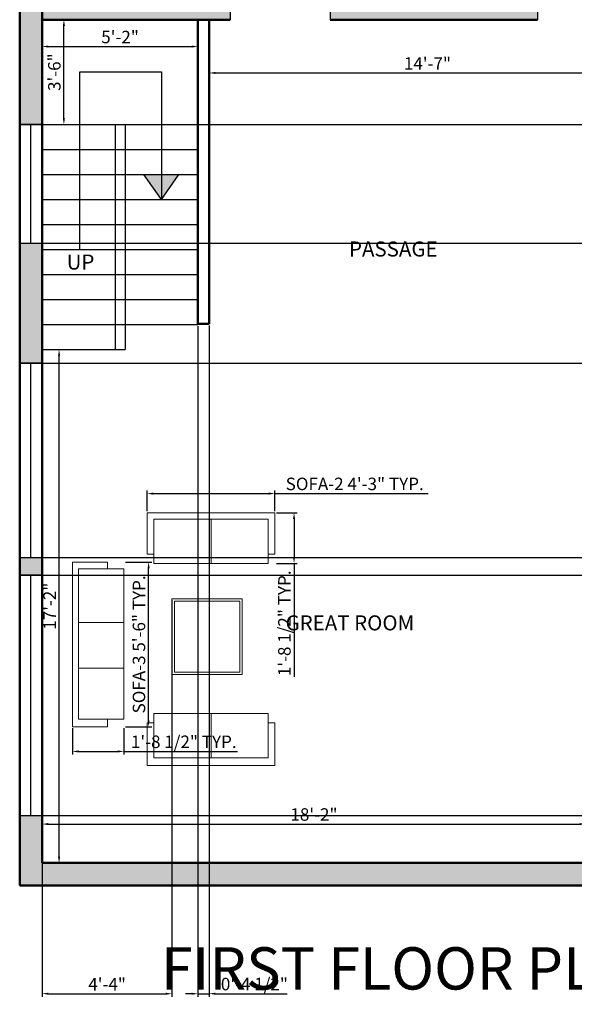
# Model space of a CAD drawing. Units: inches. Extents: x 2064 to 2999, y 1440 to 2089.
# Tile 5 of 7: x 2541 to 2763, y 1440 to 1835. Entities that reach past the tile are written whole.
import ezdxf

# ---------------------------------------------------------------- set-up
doc = ezdxf.new("R2010")
doc.units = ezdxf.units.IN
for name, color, linetype, lineweight in [('A-ANNO-DIMS', 2, 'Continuous', 18), ('A-ANNO-TEXT', 3, 'Continuous', 18), ('A-AREA-IDEN', 7, 'Continuous', 18), ('A-DOOR', 4, 'Continuous', 25), ('A-FLOR-STRS', 2, 'Continuous', 25), ('A-FURN', 8, 'Continuous', 18), ('A-GLAZ', 3, 'Continuous', 25), ('A-WALL', 7, 'Continuous', 50), ('A-WALL-PATT', 8, 'Continuous', 13)]:
    doc.layers.add(name, color=color, linetype=linetype, lineweight=lineweight)
doc.styles.get("Standard").update_dxf_attribs({"font": 'arial.ttf'})
doc.dimstyles.new('ISO-25', dxfattribs={"dimtxt": 5, "dimasz": 2.5, "dimexe": 1.25, "dimexo": 0.625, "dimtad": 1, "dimdec": 0, "dimlunit": 4, "dimtxsty": 'Standard', "dimcen": 2.5, "dimadec": 0, "dimazin": 0, "dimtfac": 1, "dimtdec": 0, "dimtmove": 0, "dimatfit": 3, "dimfxl": 1, "dimarcsym": 0})

# ---------------------------------------------------------------- blocks, each defined once
blk = doc.blocks.new('*U2')
for p, q in [((0, 0), (0, -6)), ((40, 0), (40, -6))]:
    blk.add_line(p, q)
blk.add_lwpolyline([(0, 0), (0, 40), (1.75, 40), (1.75, 0)], close=True)
blk.add_arc((0, 0), 40, 0, 90)
blk = doc.blocks.new('*D31')
at = {"layer": 'A-ANNO-DIMS', "color": 0, "lineweight": -2, "transparency": 16777216}
for p, q in [((2549.87, 1497.7), (2549.87, 1513.87)), ((2767.37, 1497.7), (2767.37, 1513.87)), ((2552.37, 1512.62), (2764.87, 1512.62))]:
    blk.add_line(p, q, dxfattribs=at)
at = {"layer": 'A-ANNO-DIMS', "color": 0, "transparency": 16777216}
for points in [[(2552.37, 1513.04), (2552.37, 1512.2), (2549.87, 1512.62)], [(2764.87, 1513.04), (2764.87, 1512.2), (2767.37, 1512.62)]]:
    blk.add_solid(points, dxfattribs=at)
at = {"layer": 'Defpoints', "color": 0, "transparency": 16777216}
for p in [(2767.37, 1512.62), (2549.87, 1497.07), (2767.37, 1497.07)]:
    blk.add_point(p, dxfattribs=at)
at = {"layer": 'A-ANNO-DIMS', "color": 0, "transparency": 16777216, "insert": (2658.62, 1515.8), "char_height": 5, "attachment_point": 5}
blk.add_mtext('18\'-2"', dxfattribs=at)
blk = doc.blocks.new('*D32')
at = {"layer": 'A-ANNO-DIMS', "color": 0, "lineweight": -2, "transparency": 16777216}
for p, q in [((2550.5, 1702.57), (2557.87, 1702.57)), ((2556.62, 1499.57), (2556.62, 1700.07)), ((2550.5, 1497.07), (2557.87, 1497.07))]:
    blk.add_line(p, q, dxfattribs=at)
at = {"layer": 'A-ANNO-DIMS', "color": 0, "transparency": 16777216}
for points in [[(2556.21, 1700.07), (2557.04, 1700.07), (2556.62, 1702.57)], [(2556.21, 1499.57), (2557.04, 1499.57), (2556.62, 1497.07)]]:
    blk.add_solid(points, dxfattribs=at)
at = {"layer": 'Defpoints', "color": 0, "transparency": 16777216}
for p in [(2549.87, 1702.57), (2556.62, 1702.57), (2549.87, 1497.07)]:
    blk.add_point(p, dxfattribs=at)
at = {"layer": 'A-ANNO-DIMS', "color": 0, "transparency": 16777216, "insert": (2553.49, 1599.82), "char_height": 5, "attachment_point": 5, "rotation": 90}
blk.add_mtext('17\'-2"', dxfattribs=at)
blk = doc.blocks.new('*D33')
at = {"layer": 'A-ANNO-DIMS', "color": 0, "lineweight": -2, "transparency": 16777216}
for p, q in [((2616.69, 1833.95), (2616.69, 1812)), ((2791.37, 1833.95), (2791.37, 1812)), ((2619.19, 1813.25), (2788.87, 1813.25))]:
    blk.add_line(p, q, dxfattribs=at)
at = {"layer": 'A-ANNO-DIMS', "color": 0, "transparency": 16777216}
for points in [[(2619.19, 1813.67), (2619.19, 1812.84), (2616.69, 1813.25)], [(2788.87, 1813.67), (2788.87, 1812.84), (2791.37, 1813.25)]]:
    blk.add_solid(points, dxfattribs=at)
at = {"layer": 'Defpoints', "color": 0, "transparency": 16777216}
for p in [(2616.69, 1834.57), (2791.37, 1834.57), (2791.37, 1813.25)]:
    blk.add_point(p, dxfattribs=at)
at = {"layer": 'A-ANNO-DIMS', "color": 0, "transparency": 16777216, "insert": (2704.03, 1816.39), "char_height": 5, "attachment_point": 5}
blk.add_mtext('14\'-7"', dxfattribs=at)
blk = doc.blocks.new('*D34')
at = {"layer": 'A-ANNO-DIMS', "color": 0, "lineweight": -2, "transparency": 16777216}
for p, q in [((2549.87, 1833.95), (2549.87, 1822.57)), ((2612.19, 1833.95), (2612.19, 1822.57)), ((2552.37, 1823.82), (2609.69, 1823.82))]:
    blk.add_line(p, q, dxfattribs=at)
at = {"layer": 'A-ANNO-DIMS', "color": 0, "transparency": 16777216}
for points in [[(2552.37, 1824.24), (2552.37, 1823.4), (2549.87, 1823.82)], [(2609.69, 1824.24), (2609.69, 1823.4), (2612.19, 1823.82)]]:
    blk.add_solid(points, dxfattribs=at)
at = {"layer": 'Defpoints', "color": 0, "transparency": 16777216}
for p in [(2549.87, 1834.57), (2612.19, 1834.57), (2612.19, 1823.82)]:
    blk.add_point(p, dxfattribs=at)
at = {"layer": 'A-ANNO-DIMS', "color": 0, "transparency": 16777216, "insert": (2581.03, 1827), "char_height": 5, "attachment_point": 5}
blk.add_mtext('5\'-2"', dxfattribs=at)
blk = doc.blocks.new('*D35')
at = {"layer": 'A-ANNO-DIMS', "color": 0, "lineweight": -2, "transparency": 16777216}
for p, q in [((2550.5, 1834.57), (2559.81, 1834.57)), ((2558.56, 1795.07), (2558.56, 1832.07)), ((2550.5, 1792.57), (2559.81, 1792.57))]:
    blk.add_line(p, q, dxfattribs=at)
at = {"layer": 'A-ANNO-DIMS', "color": 0, "transparency": 16777216}
for points in [[(2558.15, 1832.07), (2558.98, 1832.07), (2558.56, 1834.57)], [(2558.15, 1795.07), (2558.98, 1795.07), (2558.56, 1792.57)]]:
    blk.add_solid(points, dxfattribs=at)
at = {"layer": 'Defpoints', "color": 0, "transparency": 16777216}
for p in [(2549.87, 1834.57), (2558.56, 1834.57), (2549.87, 1792.57)]:
    blk.add_point(p, dxfattribs=at)
at = {"layer": 'A-ANNO-DIMS', "color": 0, "transparency": 16777216, "insert": (2555.38, 1813.57), "char_height": 5, "attachment_point": 5, "rotation": 90}
blk.add_mtext('3\'-6"', dxfattribs=at)
blk = doc.blocks.new('SOFA-2')
for p, q in [((25.58, 20.31), (25.58, 2.6)), ((2.71, 16.54), (0, 16.54)), ((0, 16.54), (0, 0)), ((51.13, 16.54), (48.46, 16.54)), ((51.13, 0), (51.13, 16.54)), ((0, 0), (51.13, 0))]:
    blk.add_line(p, q)
blk.add_lwpolyline([(2.71, 2.6), (48.46, 2.6), (48.46, 20.31), (2.71, 20.31)], close=True)
blk = doc.blocks.new('SOFA-3')
for p, q in [((0, 0), (0, 65.92)), ((0, 65.92), (14.01, 65.92)), ((14.01, 65.92), (14.01, 63.25)), ((20.61, 41.74), (2.39, 41.74)), ((20.61, 23.49), (2.39, 23.49)), ((14.01, 3.1), (14.01, 0)), ((14.01, 0), (0, 0))]:
    blk.add_line(p, q)
blk.add_lwpolyline([(2.39, 3.1), (20.61, 3.1), (20.61, 63.25), (2.39, 63.25)], close=True)
blk = doc.blocks.new('COFFEE-TABLE')
for points in [[(0, 0), (28.15, 0), (28.15, 30.4), (0, 30.4)], [(1, 1), (27.15, 1), (27.15, 29.4), (1, 29.4)]]:
    blk.add_lwpolyline(points, close=True)
blk = doc.blocks.new('*D51')
at = {"layer": 'A-ANNO-DIMS', "color": 0, "lineweight": -2, "transparency": 16777216}
for p, q in [((2591.86, 1637.86), (2591.86, 1646.15)), ((2594.36, 1644.9), (2640.49, 1644.9)), ((2642.99, 1637.86), (2642.99, 1646.15)), ((2642.99, 1644.9), (2704.36, 1644.9))]:
    blk.add_line(p, q, dxfattribs=at)
at = {"layer": 'A-ANNO-DIMS', "color": 0, "transparency": 16777216}
for points in [[(2594.36, 1645.32), (2594.36, 1644.49), (2591.86, 1644.9)], [(2640.49, 1645.32), (2640.49, 1644.49), (2642.99, 1644.9)]]:
    blk.add_solid(points, dxfattribs=at)
at = {"layer": 'Defpoints', "color": 0, "transparency": 16777216}
for p in [(2642.99, 1644.9), (2591.86, 1637.24), (2642.99, 1637.24)]:
    blk.add_point(p, dxfattribs=at)
at = {"layer": 'A-ANNO-DIMS', "color": 0, "transparency": 16777216, "insert": (2674.92, 1648.12), "char_height": 5, "attachment_point": 5}
blk.add_mtext('SOFA-2 4\'-3" TYP.', dxfattribs=at)
blk = doc.blocks.new('*D52')
at = {"layer": 'A-ANNO-DIMS', "color": 0, "lineweight": -2, "transparency": 16777216}
for p, q in [((2643.61, 1637.24), (2651.9, 1637.24)), ((2650.65, 1634.74), (2650.65, 1619.43)), ((2643.61, 1616.93), (2651.9, 1616.93)), ((2650.65, 1616.93), (2650.65, 1571.52))]:
    blk.add_line(p, q, dxfattribs=at)
at = {"layer": 'A-ANNO-DIMS', "color": 0, "transparency": 16777216}
for points in [[(2650.24, 1634.74), (2651.07, 1634.74), (2650.65, 1637.24)], [(2650.24, 1619.43), (2651.07, 1619.43), (2650.65, 1616.93)]]:
    blk.add_solid(points, dxfattribs=at)
at = {"layer": 'Defpoints', "color": 0, "transparency": 16777216}
for p in [(2642.99, 1637.24), (2642.99, 1616.93), (2650.65, 1616.93)]:
    blk.add_point(p, dxfattribs=at)
at = {"layer": 'A-ANNO-DIMS', "color": 0, "transparency": 16777216, "insert": (2647.44, 1592.97), "char_height": 5, "attachment_point": 5, "rotation": 90}
blk.add_mtext('1\'-8 1/2" TYP.', dxfattribs=at)
blk = doc.blocks.new('*D53')
at = {"layer": 'A-ANNO-DIMS', "color": 0, "lineweight": -2, "transparency": 16777216}
for p, q in [((2583.19, 1617.49), (2593.71, 1617.49)), ((2592.46, 1554.07), (2592.46, 1614.99)), ((2583.19, 1551.57), (2593.71, 1551.57))]:
    blk.add_line(p, q, dxfattribs=at)
at = {"layer": 'A-ANNO-DIMS', "color": 0, "transparency": 16777216}
for points in [[(2592.04, 1614.99), (2592.87, 1614.99), (2592.46, 1617.49)], [(2592.04, 1554.07), (2592.87, 1554.07), (2592.46, 1551.57)]]:
    blk.add_solid(points, dxfattribs=at)
at = {"layer": 'Defpoints', "color": 0, "transparency": 16777216}
for p in [(2582.57, 1617.49), (2592.46, 1617.49), (2582.57, 1551.57)]:
    blk.add_point(p, dxfattribs=at)
at = {"layer": 'A-ANNO-DIMS', "color": 0, "transparency": 16777216, "insert": (2589.24, 1584.53), "char_height": 5, "attachment_point": 5, "rotation": 90}
blk.add_mtext('SOFA-3 5\'-6" TYP.', dxfattribs=at)
blk = doc.blocks.new('*D54')
at = {"layer": 'A-ANNO-DIMS', "color": 0, "lineweight": -2, "transparency": 16777216}
for p, q in [((2561.96, 1550.95), (2561.96, 1540.44)), ((2582.57, 1550.95), (2582.57, 1540.44)), ((2564.46, 1541.69), (2580.07, 1541.69)), ((2582.57, 1541.69), (2627.98, 1541.69))]:
    blk.add_line(p, q, dxfattribs=at)
at = {"layer": 'A-ANNO-DIMS', "color": 0, "transparency": 16777216}
for points in [[(2564.46, 1542.1), (2564.46, 1541.27), (2561.96, 1541.69)], [(2580.07, 1542.1), (2580.07, 1541.27), (2582.57, 1541.69)]]:
    blk.add_solid(points, dxfattribs=at)
at = {"layer": 'Defpoints', "color": 0, "transparency": 16777216}
for p in [(2561.96, 1551.57), (2582.57, 1551.57), (2582.57, 1541.69)]:
    blk.add_point(p, dxfattribs=at)
at = {"layer": 'A-ANNO-DIMS', "color": 0, "transparency": 16777216, "insert": (2606.52, 1544.9), "char_height": 5, "attachment_point": 5}
blk.add_mtext('1\'-8 1/2" TYP.', dxfattribs=at)
blk = doc.blocks.new('*D92')
at = {"layer": 'A-ANNO-DIMS', "color": 0, "lineweight": -2, "transparency": 16777216}
for p, q in [((2541.5, 1861.72), (2996.47, 1861.72)), ((2995.22, 1859.22), (2995.22, 1795.07)), ((2541.5, 1792.57), (2996.47, 1792.57))]:
    blk.add_line(p, q, dxfattribs=at)
at = {"layer": 'A-ANNO-DIMS', "color": 0, "transparency": 16777216}
for points in [[(2994.81, 1859.22), (2995.64, 1859.22), (2995.22, 1861.72)], [(2994.81, 1795.07), (2995.64, 1795.07), (2995.22, 1792.57)]]:
    blk.add_solid(points, dxfattribs=at)
at = {"layer": 'Defpoints', "color": 0, "transparency": 16777216}
for p in [(2540.87, 1861.72), (2540.87, 1792.57), (2995.22, 1792.57)]:
    blk.add_point(p, dxfattribs=at)
at = {"layer": 'A-ANNO-DIMS', "color": 0, "transparency": 16777216, "insert": (2992.05, 1827.15), "char_height": 5, "attachment_point": 5, "rotation": 90}
blk.add_mtext('5\'-9"', dxfattribs=at)
blk = doc.blocks.new('*D93')
at = {"layer": 'A-ANNO-DIMS', "color": 0, "lineweight": -2, "transparency": 16777216}
for p, q in [((2541.5, 1745.09), (2996.47, 1745.09)), ((2995.22, 1742.59), (2995.22, 1699.57)), ((2541.5, 1697.07), (2996.47, 1697.07))]:
    blk.add_line(p, q, dxfattribs=at)
at = {"layer": 'A-ANNO-DIMS', "color": 0, "transparency": 16777216}
for points in [[(2994.81, 1742.59), (2995.64, 1742.59), (2995.22, 1745.09)], [(2994.81, 1699.57), (2995.64, 1699.57), (2995.22, 1697.07)]]:
    blk.add_solid(points, dxfattribs=at)
at = {"layer": 'Defpoints', "color": 0, "transparency": 16777216}
for p in [(2540.87, 1745.09), (2540.87, 1697.07), (2995.22, 1697.07)]:
    blk.add_point(p, dxfattribs=at)
at = {"layer": 'A-ANNO-DIMS', "color": 0, "transparency": 16777216, "insert": (2992.05, 1721.08), "char_height": 5, "attachment_point": 5, "rotation": 90}
blk.add_mtext('4\'-0"', dxfattribs=at)
blk = doc.blocks.new('*D94')
at = {"layer": 'A-ANNO-DIMS', "color": 0, "lineweight": -2, "transparency": 16777216}
for p, q in [((2541.5, 1619.25), (2996.47, 1619.25)), ((2995.22, 1616.75), (2995.22, 1614.76)), ((2541.5, 1612.26), (2996.47, 1612.26)), ((2995.22, 1612.26), (2995.22, 1595.22))]:
    blk.add_line(p, q, dxfattribs=at)
at = {"layer": 'A-ANNO-DIMS', "color": 0, "transparency": 16777216}
for points in [[(2994.81, 1616.75), (2995.64, 1616.75), (2995.22, 1619.25)], [(2994.81, 1614.76), (2995.64, 1614.76), (2995.22, 1612.26)]]:
    blk.add_solid(points, dxfattribs=at)
at = {"layer": 'Defpoints', "color": 0, "transparency": 16777216}
for p in [(2540.87, 1619.25), (2540.87, 1612.26), (2995.22, 1612.26)]:
    blk.add_point(p, dxfattribs=at)
at = {"layer": 'A-ANNO-DIMS', "color": 0, "transparency": 16777216, "insert": (2992.05, 1602.49), "char_height": 5, "attachment_point": 5, "rotation": 90}
blk.add_mtext('0\'-7"', dxfattribs=at)
blk = doc.blocks.new('*D95')
at = {"layer": 'A-ANNO-DIMS', "color": 0, "lineweight": -2, "transparency": 16777216}
for p, q in [((2541.5, 1516.02), (2996.47, 1516.02)), ((2995.22, 1513.52), (2995.22, 1490.57)), ((2541.5, 1488.07), (2996.47, 1488.07))]:
    blk.add_line(p, q, dxfattribs=at)
at = {"layer": 'A-ANNO-DIMS', "color": 0, "transparency": 16777216}
for points in [[(2994.81, 1513.52), (2995.64, 1513.52), (2995.22, 1516.02)], [(2994.81, 1490.57), (2995.64, 1490.57), (2995.22, 1488.07)]]:
    blk.add_solid(points, dxfattribs=at)
at = {"layer": 'Defpoints', "color": 0, "transparency": 16777216}
for p in [(2540.87, 1516.02), (2540.87, 1488.07), (2995.22, 1488.07)]:
    blk.add_point(p, dxfattribs=at)
at = {"layer": 'A-ANNO-DIMS', "color": 0, "transparency": 16777216, "insert": (2992.09, 1502.05), "char_height": 5, "attachment_point": 5, "rotation": 90}
blk.add_mtext('2\'-4"', dxfattribs=at)
blk = doc.blocks.new('*D98')
at = {"layer": 'A-ANNO-DIMS', "color": 0, "lineweight": -2, "transparency": 16777216}
for p, q in [((2612.19, 1711.95), (2612.19, 1443.47)), ((2616.69, 1712.16), (2616.69, 1443.47)), ((2609.69, 1444.72), (2607.19, 1444.72)), ((2612.19, 1444.72), (2616.69, 1444.72)), ((2619.19, 1444.72), (2647.88, 1444.72))]:
    blk.add_line(p, q, dxfattribs=at)
at = {"layer": 'A-ANNO-DIMS', "color": 0, "transparency": 16777216}
for points in [[(2609.69, 1445.14), (2609.69, 1444.3), (2612.19, 1444.72)], [(2619.19, 1445.14), (2619.19, 1444.3), (2616.69, 1444.72)]]:
    blk.add_solid(points, dxfattribs=at)
at = {"layer": 'Defpoints', "color": 0, "transparency": 16777216}
for p in [(2612.19, 1712.57), (2616.69, 1712.78), (2616.69, 1444.72)]:
    blk.add_point(p, dxfattribs=at)
at = {"layer": 'A-ANNO-DIMS', "color": 0, "transparency": 16777216, "insert": (2634.78, 1447.93), "char_height": 5, "attachment_point": 5}
blk.add_mtext('0\'-4 1/2"', dxfattribs=at)
blk = doc.blocks.new('*D109')
at = {"layer": 'A-ANNO-DIMS', "color": 0, "lineweight": -2, "transparency": 16777216}
for p, q in [((2549.87, 1611.64), (2549.87, 1443.47)), ((2601.8, 1602.21), (2601.8, 1443.47)), ((2552.37, 1444.72), (2599.3, 1444.72))]:
    blk.add_line(p, q, dxfattribs=at)
at = {"layer": 'A-ANNO-DIMS', "color": 0, "transparency": 16777216}
for points in [[(2552.37, 1445.14), (2552.37, 1444.3), (2549.87, 1444.72)], [(2599.3, 1445.14), (2599.3, 1444.3), (2601.8, 1444.72)]]:
    blk.add_solid(points, dxfattribs=at)
at = {"layer": 'Defpoints', "color": 0, "transparency": 16777216}
for p in [(2549.87, 1612.26), (2601.8, 1602.84), (2601.8, 1444.72)]:
    blk.add_point(p, dxfattribs=at)
at = {"layer": 'A-ANNO-DIMS', "color": 0, "transparency": 16777216, "insert": (2575.84, 1447.85), "char_height": 5, "attachment_point": 5}
blk.add_mtext('4\'-4"', dxfattribs=at)

msp = doc.modelspace()

# ---------------------------------------------------------------- hatches: boundary and pattern name
at = {"layer": 'A-FLOR-STRS'}
h = msp.add_hatch(color=256, dxfattribs=at)
h.dxf.hatch_style = 1
h.paths.add_polyline_path([(2597.57, 1772.57), (2590.58, 1772.57), (2597.57, 1762.57)])
h.paths.add_polyline_path([(2604.57, 1772.57), (2597.57, 1772.57), (2597.57, 1762.57)])
at = {"layer": 'A-WALL-PATT'}
h = msp.add_hatch(color=256, dxfattribs=at)
h.dxf.hatch_style = 1
h.paths.add_polyline_path([(2574.52, 1968.07), (2540.87, 1968.07), (2540.87, 1930.52), (2549.87, 1930.52), (2549.87, 1959.07), (2574.52, 1959.07)])
h.paths.add_polyline_path([(2687.51, 1968.07), (2643.06, 1968.07), (2643.06, 1959.07), (2669.87, 1959.07), (2687.51, 1959.07)])
h.paths.add_polyline_path([(2900.87, 1968.07), (2728.11, 1968.07), (2728.11, 1959.07), (2740.37, 1959.07), (2891.87, 1959.07), (2891.87, 1930.52), (2900.87, 1930.52)])
h.paths.add_polyline_path([(2744.87, 1959.07), (2740.37, 1959.07), (2740.37, 1839.07), (2674.37, 1839.07), (2674.37, 1959.07), (2669.87, 1959.07), (2669.87, 1892.49), (2669.87, 1839.07), (2665.15, 1839.07), (2665.15, 1834.57), (2674.37, 1834.57), (2744.87, 1834.57), (2748.11, 1834.57), (2748.11, 1839.07), (2744.87, 1839.07)])
h.paths.add_polyline_path([(2549.87, 1834.57), (2549.87, 1861.72), (2540.87, 1861.72), (2540.87, 1792.57), (2549.87, 1792.57)])
h.paths.add_polyline_path([(2625.15, 1839.07), (2549.87, 1839.07), (2549.87, 1834.57), (2625.15, 1834.57)])
h.paths.add_polyline_path([(2900.87, 1861.72), (2891.87, 1861.72), (2891.87, 1810.41), (2900.87, 1810.41)])
h.paths.add_polyline_path([(2891.87, 1839.07), (2788.11, 1839.07), (2788.11, 1834.57), (2891.87, 1834.57)])
h.paths.add_polyline_path([(2549.87, 1745.09), (2540.87, 1745.09), (2540.87, 1697.07), (2549.87, 1697.07)])
h.paths.add_polyline_path([(2549.87, 1619.25), (2540.87, 1619.25), (2540.87, 1612.26), (2549.87, 1612.26)], flags=17)
h.paths.add_polyline_path([(2549.87, 1516.02), (2540.87, 1516.02), (2540.87, 1488.07), (2900.87, 1488.07), (2900.87, 1682.51), (2891.87, 1682.51), (2891.87, 1497.07), (2549.87, 1497.07)])
h.paths.add_polyline_path([(2771.87, 1575.08), (2767.37, 1575.08), (2767.37, 1497.07), (2771.87, 1497.07)], flags=17)
h.paths.add_polyline_path([(2771.87, 1708.85), (2767.37, 1708.85), (2767.37, 1633.57), (2771.87, 1633.57), (2771.87, 1638.07)])
h.paths.add_polyline_path([(2891.87, 1638.07), (2780.13, 1638.07), (2771.87, 1638.07), (2771.87, 1633.57), (2891.87, 1633.57)], flags=17)
h.paths.add_polyline_path([(2771.87, 1633.57), (2767.37, 1633.57), (2767.37, 1615.08), (2771.87, 1615.08)], flags=17)
h.paths.add_polyline_path([(2900.87, 1784.26), (2891.87, 1784.26), (2891.87, 1751.31), (2900.87, 1751.31)])
h.paths.add_polyline_path([(2795.87, 1834.57), (2791.37, 1834.57), (2791.37, 1830.13), (2795.87, 1830.13)])
h.paths.add_polyline_path([(2805.14, 1771.92), (2830.56, 1771.92), (2830.56, 1784.32), (2805.14, 1784.32)], flags=9)
h.paths.add_polyline_path([(2805.18, 1686.98), (2865.14, 1686.98), (2865.14, 1699.38), (2805.18, 1699.38)], flags=9)
h.paths.add_polyline_path([(2801, 1552.43), (2850.22, 1552.43), (2850.22, 1564.83), (2801, 1564.83)], flags=25)
h.paths.add_polyline_path([(2645.3, 1586.75), (2705.73, 1586.75), (2705.73, 1599.14), (2645.3, 1599.14)], flags=25)
h.paths.add_polyline_path([(2670.49, 1736.4), (2713.67, 1736.4), (2713.67, 1748.79), (2670.49, 1748.79)], flags=9)
h.paths.add_polyline_path([(2795.9, 1895.95), (2857.73, 1895.95), (2857.73, 1908.34), (2795.9, 1908.34)], flags=9)
h.paths.add_polyline_path([(2565.91, 1921.55), (2649.69, 1921.55), (2649.69, 1933.95), (2565.91, 1933.95)], flags=9)

# ---------------------------------------------------------------- linework, layer by layer
at = {"layer": 'A-FLOR-STRS'}
for p, q in [((2564.92, 1742.57), (2564.92, 1813.68)), ((2564.92, 1813.68), (2597.57, 1813.68)), ((2597.57, 1813.68), (2597.57, 1762.57)), ((2549.87, 1792.57), (2612.19, 1792.57)), ((2579.03, 1792.57), (2579.03, 1712.78)), ((2583.03, 1792.57), (2583.03, 1712.78)), ((2549.87, 1782.57), (2612.19, 1782.57)), ((2549.87, 1772.57), (2612.19, 1772.57)), ((2597.57, 1762.57), (2590.58, 1772.57)), ((2597.57, 1762.57), (2604.57, 1772.57)), ((2549.87, 1762.57), (2612.19, 1762.57)), ((2549.87, 1752.57), (2612.19, 1752.57)), ((2549.87, 1742.57), (2612.19, 1742.57)), ((2549.87, 1732.57), (2612.19, 1732.57)), ((2549.87, 1722.57), (2612.19, 1722.57)), ((2549.87, 1712.57), (2612.19, 1712.57)), ((2579.03, 1712.78), (2579.03, 1702.57)), ((2583.03, 1712.78), (2583.03, 1702.57)), ((2549.87, 1702.57), (2583.03, 1702.57))]:
    msp.add_line(p, q, dxfattribs=at)
at = {"layer": 'A-FURN'}
for p, q in [((2617.44, 1556.88), (2617.44, 1539.17)), ((2594.57, 1553.11), (2591.86, 1553.11)), ((2591.86, 1553.11), (2591.86, 1536.1)), ((2642.99, 1553.11), (2640.31, 1553.11)), ((2642.99, 1536.1), (2642.99, 1553.11)), ((2591.86, 1536.1), (2642.99, 1536.1))]:
    msp.add_line(p, q, dxfattribs=at)
msp.add_lwpolyline([(2594.57, 1539.17), (2640.31, 1539.17), (2640.31, 1556.88), (2594.57, 1556.88)], close=True, dxfattribs=at)
at = {"layer": 'A-GLAZ'}
for p, q in [((2545.37, 1745.09), (2545.37, 1792.57)), ((2545.37, 1619.25), (2545.37, 1697.07)), ((2545.37, 1516.02), (2545.37, 1612.26))]:
    msp.add_line(p, q, dxfattribs=at)
for points in [[(2540.87, 1745.09), (2549.87, 1745.09), (2549.87, 1792.57), (2540.87, 1792.57)], [(2540.87, 1619.25), (2549.87, 1619.25), (2549.87, 1697.07), (2540.87, 1697.07)], [(2540.87, 1516.02), (2549.87, 1516.02), (2549.87, 1612.26), (2540.87, 1612.26)]]:
    msp.add_lwpolyline(points, close=True, dxfattribs=at)
at = {"layer": 'A-WALL'}
for p, q in [((2540.87, 1488.07), (2540.87, 1968.07)), ((2549.87, 1497.07), (2549.87, 1959.07)), ((2625.15, 1834.57), (2549.87, 1834.57)), ((2549.87, 1834.57), (2549.87, 1792.57)), ((2612.19, 1712.78), (2612.19, 1834.57)), ((2616.69, 1834.57), (2616.69, 1712.78)), ((2674.37, 1834.57), (2665.15, 1834.57)), ((2744.87, 1834.57), (2674.37, 1834.57)), ((2744.87, 1834.57), (2748.11, 1834.57)), ((2616.69, 1712.78), (2612.19, 1712.78)), ((2549.87, 1497.07), (2549.87, 1697.07)), ((2891.87, 1497.07), (2549.87, 1497.07)), ((2900.87, 1488.07), (2540.87, 1488.07))]:
    msp.add_line(p, q, dxfattribs=at)

# ---------------------------------------------------------------- block references
at = {"layer": 'A-DOOR', "xscale": -1}
msp.add_blockref('*U2', (2665.15, 1840.57), dxfattribs=at)
at = {"layer": 'A-DOOR'}
msp.add_blockref('*U2', (2748.11, 1840.57), dxfattribs=at)
at = {"layer": 'A-FURN', "extrusion": (0, 0, -1), "zscale": -1, "rotation": 180}
msp.add_blockref('SOFA-2', (-2591.86, 1637.24), dxfattribs=at)
at = {"layer": 'A-FURN'}
for name, p in [('SOFA-3', (2561.96, 1551.57)), ('COFFEE-TABLE', (2601.8, 1572.43))]:
    msp.add_blockref(name, p, dxfattribs=at)

# ---------------------------------------------------------------- texts
at = {"layer": 'A-ANNO-TEXT', "insert": (2597.31, 1463.31), "char_height": 16.9292, "attachment_point": 1}
msp.add_mtext_dynamic_manual_height_columns('FIRST FLOOR PLAN', width=429.6774, gutter_width=84.65, heights=[17.52], dxfattribs=at)
at = {"layer": 'A-AREA-IDEN', "char_height": 6.015, "attachment_point": 1}
for s, insert in [('PASSAGE', (2672.64, 1745.8)), ('UP', (2559.65, 1740.57)), ('GREAT ROOM', (2647.25, 1596.15))]:
    msp.add_mtext_dynamic_manual_height_columns(s, width=152.6727, gutter_width=30.08, heights=[0], dxfattribs=dict(at, insert=insert))

# ---------------------------------------------------------------- dimensions: what is measured, and where the dimension line sits
at = {"layer": 'A-ANNO-DIMS'}
for base, p1, p2, override, picture, middle in [((2995.2249, 1792.5709), (2540.8749, 1861.7244), (2540.8749, 1792.5709), {"dimdec": 1, "dimlfac": 1, "dimrnd": 0, "dimzin": 1, "dimdsep": 46, "dimlunit": 4, "dimfrac": 2}, '*D92', (2992.0471, 1827.1477)), ((2558.56, 1834.57), (2549.87, 1792.57), (2549.87, 1834.57), {"dimclrd": 0, "dimclre": 0, "dimclrt": 0}, '*D35', (2555.38, 1813.57)), ((2995.22, 1697.07), (2540.87, 1745.09), (2540.87, 1697.07), {"dimdec": 1, "dimlfac": 1, "dimrnd": 0, "dimzin": 1, "dimdsep": 46, "dimlunit": 4, "dimfrac": 2}, '*D93', (2992.05, 1721.08)), ((2556.62443158, 1702.570928), (2549.87494438, 1497.070928), (2549.87494438, 1702.570928), {"dimclrd": 0, "dimclre": 0, "dimclrt": 0}, '*D32', (2553.48919966, 1599.820928)), ((2995.22, 1612.26), (2540.87, 1619.25), (2540.87, 1612.26), {"dimdec": 1, "dimlfac": 1, "dimrnd": 0, "dimzin": 1, "dimdsep": 46, "dimlunit": 4, "dimfrac": 2}, '*D94', (2992.05, 1602.49)), ((2995.2249, 1488.0709), (2540.8749, 1516.021), (2540.8749, 1488.0709), {"dimdec": 1, "dimlfac": 1, "dimrnd": 0, "dimzin": 1, "dimdsep": 46, "dimlunit": 4, "dimfrac": 2}, '*D95', (2992.0897, 1502.046))]:
    dim = msp.add_linear_dim(base=base, p1=p1, p2=p2, angle=90, dimstyle='ISO-25', override=override, dxfattribs=at)
    dim.commit()
    dim.dimension.update_dxf_attribs({"geometry": picture, "text_midpoint": middle})
for base, p1, p2, override, picture, middle in [((2612.19, 1823.82), (2549.87, 1834.57), (2612.19, 1834.57), {"dimclrd": 0, "dimclre": 0, "dimclrt": 0}, '*D34', (2581.03, 1827)), ((2791.37, 1813.25), (2616.69, 1834.57), (2791.37, 1834.57), {"dimclrd": 0, "dimclre": 0, "dimclrt": 0}, '*D33', (2704.03, 1816.39)), ((2616.69, 1444.72), (2612.19, 1712.57), (2616.69, 1712.78), {"dimdec": 1, "dimlfac": 1, "dimrnd": 0, "dimzin": 1, "dimdsep": 46, "dimlunit": 4, "dimfrac": 2}, '*D98', (2634.78, 1447.93)), ((2601.8, 1444.72), (2549.87, 1612.26), (2601.8, 1602.84), {"dimdec": 1, "dimlfac": 1, "dimrnd": 0, "dimzin": 1, "dimdsep": 46, "dimlunit": 4, "dimfrac": 2}, '*D109', (2575.84, 1447.85)), ((2767.37494438, 1512.62136921), (2549.87494438, 1497.070928), (2767.37494438, 1497.070928), {"dimclrd": 0, "dimclre": 0, "dimclrt": 0}, '*D31', (2658.62494438, 1515.79923415))]:
    dim = msp.add_linear_dim(base=base, p1=p1, p2=p2, dimstyle='ISO-25', override=override, dxfattribs=at)
    dim.commit()
    dim.dimension.update_dxf_attribs({"geometry": picture, "text_midpoint": middle})
for base, p1, p2, text, picture, middle in [((2642.99, 1644.9), (2591.86, 1637.24), (2642.99, 1637.24), 'SOFA-2 <> TYP.', '*D51', (2674.92, 1648.12)), ((2582.57, 1541.69), (2561.96, 1551.57), (2582.57, 1551.57), '<> TYP.', '*D54', (2606.52, 1544.9))]:
    dim = msp.add_linear_dim(base=base, p1=p1, p2=p2, text=text, dimstyle='ISO-25', override={"dimdec": 1, "dimrnd": 0, "dimzin": 1, "dimlunit": 4, "dimfrac": 2}, dxfattribs=at)
    dim.commit()
    dim.dimension.update_dxf_attribs({"geometry": picture, "text_midpoint": middle})
for base, p1, p2, angle, text, picture, middle in [((2650.65, 1616.93), (2642.99, 1637.24), (2642.99, 1616.93), 270, '<> TYP.', '*D52', (2647.44, 1592.97)), ((2592.46, 1617.49), (2582.57, 1551.57), (2582.57, 1617.49), 90, 'SOFA-3 <> TYP.', '*D53', (2589.24, 1584.53))]:
    dim = msp.add_linear_dim(base=base, p1=p1, p2=p2, angle=angle, text=text, dimstyle='ISO-25', override={"dimdec": 1, "dimrnd": 0, "dimzin": 1, "dimlunit": 4, "dimfrac": 2}, dxfattribs=at)
    dim.commit()
    dim.dimension.update_dxf_attribs({"geometry": picture, "text_midpoint": middle})

doc.saveas('drawing.dxf')
